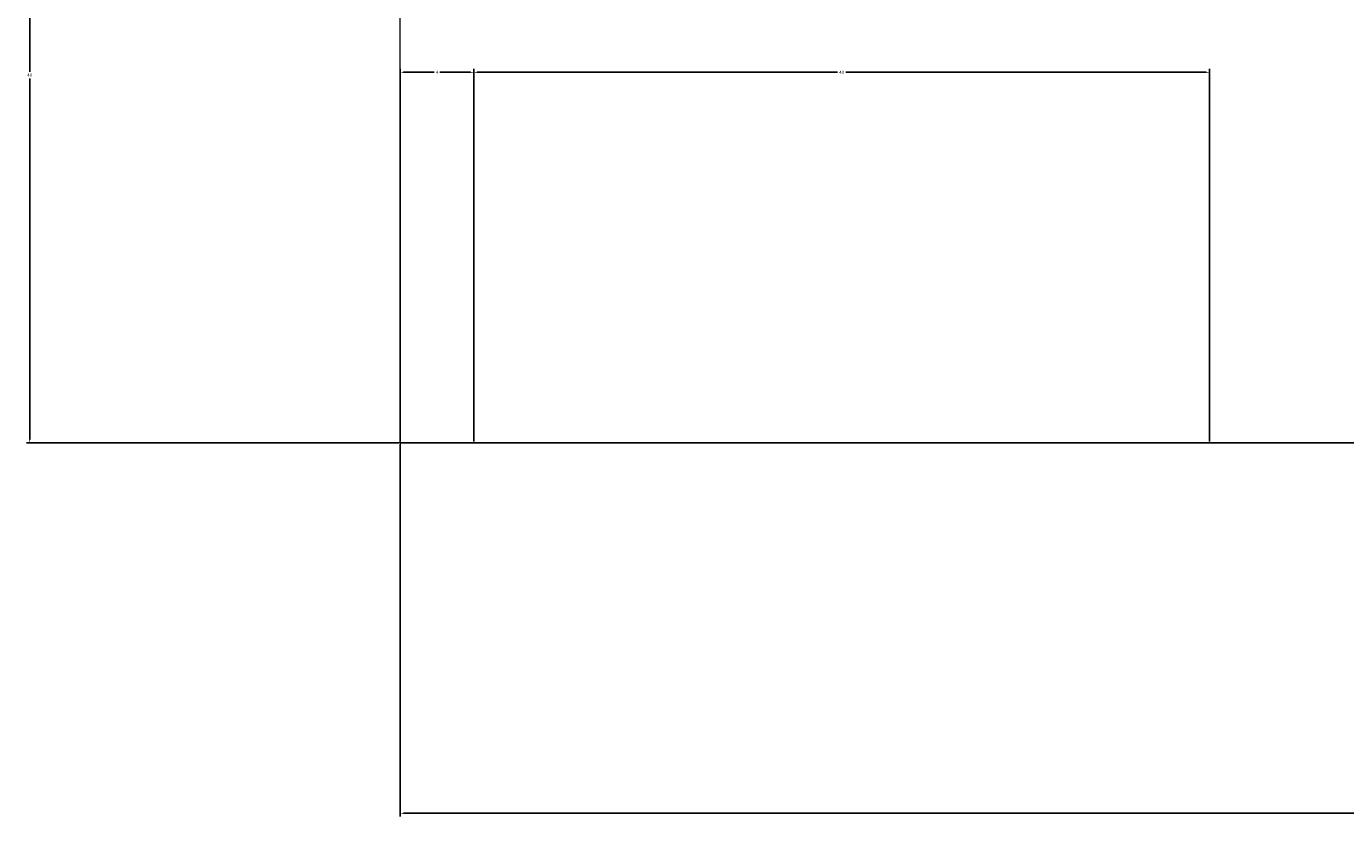
# Model space of a CAD drawing. Units: inches. Extents: x 1095 to 1408, y -20 to 240.
# Tile 1 of 8: x 1095 to 1167, y -20 to 23. Entities that reach past the tile are written whole.
import ezdxf

# ---------------------------------------------------------------- set-up
doc = ezdxf.new("R2010")
doc.units = ezdxf.units.IN
doc.header["$MEASUREMENT"] = 0
doc.layers.add('M-CONS', color=8, linetype='Continuous', lineweight=18)
doc.layers.add('M-DIMS', color=2, linetype='Continuous', lineweight=18)
doc.styles.get("Standard").update_dxf_attribs({"font": 'arial.ttf'})
doc.dimstyles.get("Standard").update_dxf_attribs({"dimtxt": 0.18, "dimasz": 0.18, "dimexe": 0.18, "dimexo": 0.0625, "dimgap": 0.09, "dimtad": 0, "dimtih": 1, "dimtoh": 1, "dimdec": 4, "dimzin": 0, "dimdsep": 46, "dimtxsty": 'Standard', "dimcen": 0.09, "dimadec": 0, "dimazin": 0, "dimtfac": 1, "dimtdec": 4, "dimtofl": 0, "dimtmove": 0, "dimatfit": 3, "dimfxl": 1, "dimtolj": 1, "dimtzin": 0, "dimarcsym": 0})

# ---------------------------------------------------------------- blocks, each defined once
blk = doc.blocks.new('*D1')
at = {"layer": 'Defpoints', "color": 0, "transparency": 16777216}
for p in [(1115.184, 0), (1387.184, 0), (1387.184, -20.15)]:
    blk.add_point(p, dxfattribs=at)
at = {"layer": 'M-DIMS', "color": 0, "lineweight": -2, "transparency": 16777216}
for p, q in [((1115.184, -0.062), (1115.184, -20.33)), ((1387.184, -0.062), (1387.184, -20.33)), ((1115.364, -20.15), (1250.894, -20.15)), ((1387.004, -20.15), (1251.473, -20.15))]:
    blk.add_line(p, q, dxfattribs=at)
at = {"layer": 'M-DIMS', "color": 0, "transparency": 16777216}
for points in [[(1115.364, -20.12), (1115.364, -20.18), (1115.184, -20.15)], [(1387.004, -20.12), (1387.004, -20.18), (1387.184, -20.15)]]:
    blk.add_solid(points, dxfattribs=at)
at = {"layer": 'M-DIMS', "color": 0, "transparency": 16777216, "insert": (1251.184, -20.15), "char_height": 0.18, "attachment_point": 5}
blk.add_mtext('\\A1;272', dxfattribs=at)
blk = doc.blocks.new('*D4')
at = {"layer": 'Defpoints', "color": 0, "transparency": 16777216}
for p in [(1095.034, 40), (1115.184, 40), (1115.184, 0)]:
    blk.add_point(p, dxfattribs=at)
at = {"layer": 'M-DIMS', "color": 0, "lineweight": -2, "transparency": 16777216}
for p, q in [((1115.121, 40), (1094.854, 40)), ((1095.034, 39.82), (1095.034, 20.182)), ((1095.034, 0.18), (1095.034, 19.818)), ((1115.121, 0), (1094.854, 0))]:
    blk.add_line(p, q, dxfattribs=at)
at = {"layer": 'M-DIMS', "color": 0, "transparency": 16777216}
for points in [[(1095.004, 39.82), (1095.064, 39.82), (1095.034, 40)], [(1095.004, 0.18), (1095.064, 0.18), (1095.034, 0)]]:
    blk.add_solid(points, dxfattribs=at)
at = {"layer": 'M-DIMS', "color": 0, "transparency": 16777216, "insert": (1095.034, 20), "char_height": 0.18, "attachment_point": 5}
blk.add_mtext('\\A1;40', dxfattribs=at)
blk = doc.blocks.new('*D13')
at = {"layer": 'Defpoints', "color": 0, "transparency": 16777216}
for p in [(1159.184, 20.15), (1119.184, 0), (1159.184, 0)]:
    blk.add_point(p, dxfattribs=at)
at = {"layer": 'M-DIMS', "color": 0, "lineweight": -2, "transparency": 16777216}
for p, q in [((1119.184, 0.062), (1119.184, 20.33)), ((1119.364, 20.15), (1138.961, 20.15)), ((1159.004, 20.15), (1139.406, 20.15)), ((1159.184, 0.062), (1159.184, 20.33))]:
    blk.add_line(p, q, dxfattribs=at)
at = {"layer": 'M-DIMS', "color": 0, "transparency": 16777216}
for points in [[(1119.364, 20.18), (1119.364, 20.12), (1119.184, 20.15)], [(1159.004, 20.18), (1159.004, 20.12), (1159.184, 20.15)]]:
    blk.add_solid(points, dxfattribs=at)
at = {"layer": 'M-DIMS', "color": 0, "transparency": 16777216, "insert": (1139.184, 20.15), "char_height": 0.18, "attachment_point": 5}
blk.add_mtext('\\A1;40', dxfattribs=at)
blk = doc.blocks.new('*D14')
at = {"layer": 'Defpoints', "color": 0, "transparency": 16777216}
for p in [(1119.184, 20.15), (1115.184, 0), (1119.184, 0)]:
    blk.add_point(p, dxfattribs=at)
at = {"layer": 'M-DIMS', "color": 0, "lineweight": -2, "transparency": 16777216}
for p, q in [((1115.184, 0.062), (1115.184, 20.33)), ((1115.364, 20.15), (1117.031, 20.15)), ((1119.004, 20.15), (1117.336, 20.15)), ((1119.184, 0.062), (1119.184, 20.33))]:
    blk.add_line(p, q, dxfattribs=at)
at = {"layer": 'M-DIMS', "color": 0, "transparency": 16777216}
for points in [[(1115.364, 20.18), (1115.364, 20.12), (1115.184, 20.15)], [(1119.004, 20.18), (1119.004, 20.12), (1119.184, 20.15)]]:
    blk.add_solid(points, dxfattribs=at)
at = {"layer": 'M-DIMS', "color": 0, "transparency": 16777216, "insert": (1117.184, 20.15), "char_height": 0.18, "attachment_point": 5}
blk.add_mtext('\\A1;4', dxfattribs=at)

msp = doc.modelspace()

# ---------------------------------------------------------------- linework, layer by layer
at = {"layer": 'M-CONS'}
msp.add_line((1115.184, 0, 397.783), (1115.184, 40, 397.783), dxfattribs=at)
at = {"layer": 'M-CONS', "extrusion": (0, -1, 0)}
for p, q in [((1159.184, 0, 397.783), (1115.184, 0, 397.783)), ((1115.184, 0, 397.783), (1115.184, 0, 357.783)), ((1115.184, 0, 357.783), (1387.184, 0, 357.783)), ((1383.184, 0, 377.783), (1119.184, 0, 377.783)), ((1119.184, 0, 377.783), (1119.184, 0, 392.783)), ((1119.184, 0, 392.783), (1159.184, 0, 392.783)), ((1159.184, 0, 392.783), (1159.184, 0, 397.783))]:
    msp.add_line(p, q, dxfattribs=at)

# ---------------------------------------------------------------- dimensions: what is measured, and where the dimension line sits
at = {"layer": 'M-DIMS'}
dim = msp.add_linear_dim(base=(1095.034, 40), p1=(1115.184, 0), p2=(1115.184, 40), angle=90, dimstyle='Standard', override={"dimdec": 0, "dimlfac": 1, "dimrnd": 0, "dimzin": 0, "dimdsep": 46, "dimlunit": 2}, dxfattribs=at)
dim.commit()
dim.dimension.update_dxf_attribs({"geometry": '*D4', "text_midpoint": (1095.034, 20)})
for base, p1, p2, picture, middle in [((1119.184, 20.15), (1115.184, 0), (1119.184, 0), '*D14', (1117.184, 20.15)), ((1159.184, 20.15), (1119.184, 0), (1159.184, 0), '*D13', (1139.184, 20.15)), ((1387.184, -20.15), (1115.184, 0), (1387.184, 0), '*D1', (1251.184, -20.15))]:
    dim = msp.add_linear_dim(base=base, p1=p1, p2=p2, dimstyle='Standard', override={"dimdec": 0, "dimlfac": 1, "dimrnd": 0, "dimzin": 0, "dimdsep": 46, "dimlunit": 2}, dxfattribs=at)
    dim.commit()
    dim.dimension.update_dxf_attribs({"geometry": picture, "text_midpoint": middle})

doc.saveas('drawing.dxf')
